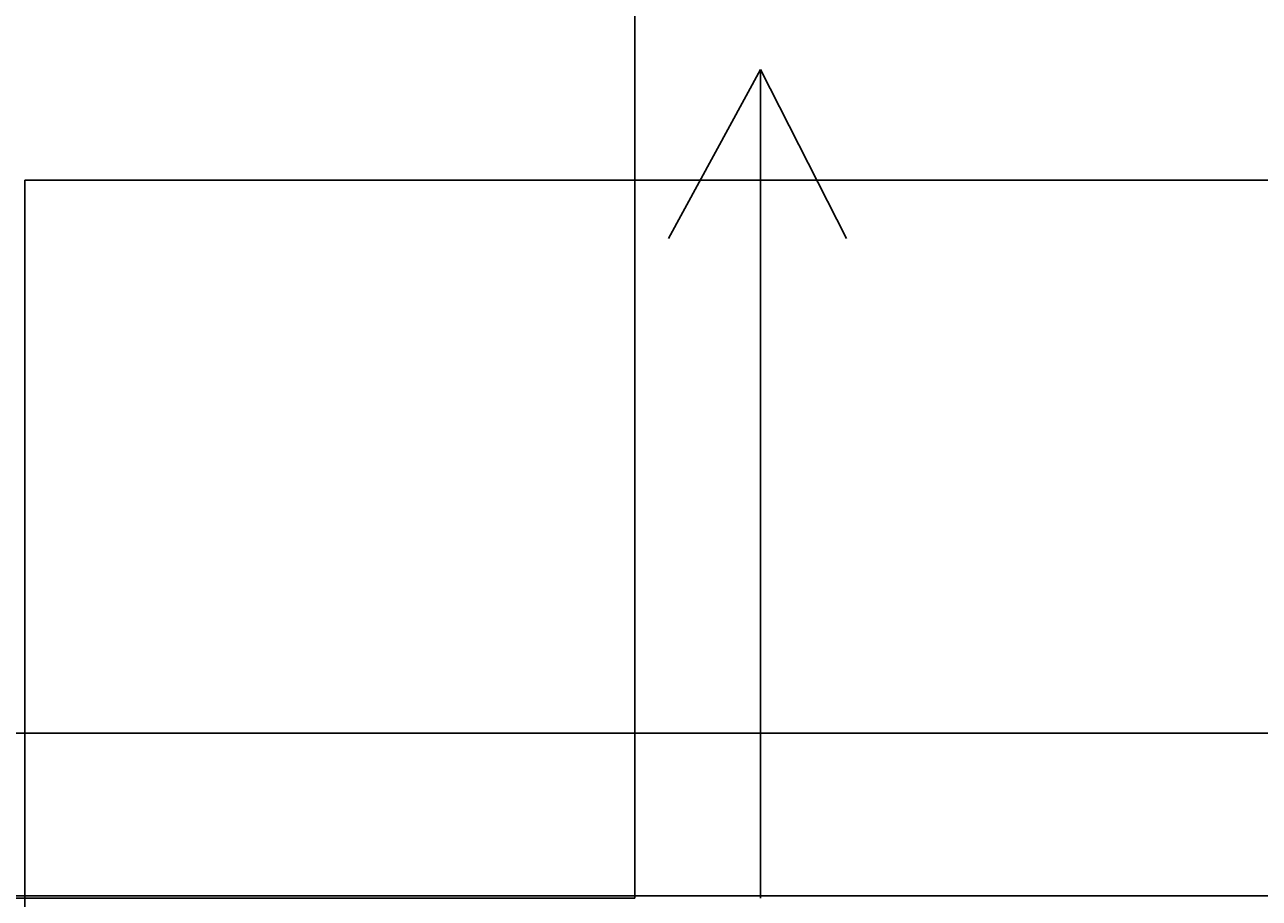
# Model space of a CAD drawing. Units: inches. Extents: x 35362 to 73946, y 43607 to 67532.
# Tile 134 of 134: x 67327 to 69338, y 60122 to 61547. Entities that reach past the tile are written whole.
import ezdxf

# ---------------------------------------------------------------- set-up
doc = ezdxf.new("R2010")
doc.units = ezdxf.units.IN
doc.header["$MEASUREMENT"] = 0
doc.layers.add('A-ANNO-DIMS', color=2, linetype='Continuous', lineweight=18)
doc.layers.add('E-SYMB', color=1, linetype='Continuous', lineweight=25)
doc.styles.get("Standard").update_dxf_attribs({"font": 'arial.ttf'})
doc.dimstyles.get("Standard").update_dxf_attribs({"dimtxt": 0.18, "dimasz": 0.18, "dimexe": 0.18, "dimexo": 0.0625, "dimgap": 0.09, "dimtad": 0, "dimtih": 1, "dimtoh": 1, "dimdec": 4, "dimzin": 0, "dimdsep": 46, "dimtxsty": 'Standard', "dimcen": 0.09, "dimadec": 0, "dimazin": 0, "dimtfac": 1, "dimtdec": 4, "dimtofl": 0, "dimtmove": 0, "dimatfit": 3, "dimfxl": 1, "dimtolj": 1, "dimtzin": 0, "dimarcsym": 0})

# ---------------------------------------------------------------- blocks, each defined once
blk = doc.blocks.new('PWR-5V')
for p, q in [((149.83075954589, 1350.920325582869), (-0.0001436721213395, 1075.898385659784)), ((149.83075954589, 833.0941938853575), (149.83075954589, 1350.920325582869)), ((289.9554714129044, 1075.898385659784), (149.83075954589, 1350.920325582869)), ((149.83075954589, 416.3126341884199), (149.83075954589, 833.0941938853575)), ((149.83075954589, 416.3126341884199), (149.83075954589, 0.0003315384019515))]:
    blk.add_line(p, q)
blk = doc.blocks.new('*D8')
at = {"layer": 'A-ANNO-DIMS', "color": 0, "lineweight": -2, "transparency": 16777216}
for p, q in [((66271.28651900003, 65771.51172800003), (73945.82566600003, 65771.51172800003)), ((73945.64566600005, 65771.33172800003), (73945.64566600005, 59737.03093663782)), ((73945.64566600005, 53702.36633900002), (73945.64566600005, 59736.66713036224)), ((72185.70816600003, 53702.18633900003), (73945.82566600003, 53702.18633900003))]:
    blk.add_line(p, q, dxfattribs=at)
at = {"layer": 'A-ANNO-DIMS', "color": 0, "transparency": 16777216}
for points in [[(73945.61566600006, 65771.33172800003), (73945.67566600005, 65771.33172800003), (73945.64566600005, 65771.51172800003)], [(73945.61566600006, 53702.36633900002), (73945.67566600005, 53702.36633900002), (73945.64566600005, 53702.18633900003)]]:
    blk.add_solid(points, dxfattribs=at)
at = {"layer": 'Defpoints', "color": 0, "transparency": 16777216}
for p in [(66271.22401900003, 65771.51172800003), (73945.64566600005, 65771.51172800003), (72185.64566600003, 53702.18633900003)]:
    blk.add_point(p, dxfattribs=at)
at = {"layer": 'A-ANNO-DIMS', "color": 0, "transparency": 16777216, "insert": (73945.64566600005, 59736.84903349999), "char_height": 0.18, "attachment_point": 5}
blk.add_mtext('\\A1;12069', dxfattribs=at)
blk = doc.blocks.new('*D35')
at = {"layer": 'A-ANNO-DIMS', "color": 0, "lineweight": -2, "transparency": 16777216}
for p, q in [((61240.907336, 59185.206457), (61240.907336, 67531.691728)), ((61241.08733599999, 67531.51172799998), (64780.42646373397, 67531.51172799998)), ((68320.69076200001, 67531.51172799998), (64781.35163426603, 67531.51172799998)), ((68320.870762, 60122.408832), (68320.870762, 67531.691728))]:
    blk.add_line(p, q, dxfattribs=at)
at = {"layer": 'A-ANNO-DIMS', "color": 0, "transparency": 16777216}
for points in [[(61241.08733599999, 67531.541728), (61241.08733599999, 67531.481728), (61240.907336, 67531.51172799998)], [(68320.69076200001, 67531.541728), (68320.69076200001, 67531.481728), (68320.870762, 67531.51172799998)]]:
    blk.add_solid(points, dxfattribs=at)
at = {"layer": 'Defpoints', "color": 0, "transparency": 16777216}
for p in [(68320.870762, 67531.51172799998), (68320.870762, 60122.346332), (61240.907336, 59185.14395699999)]:
    blk.add_point(p, dxfattribs=at)
at = {"layer": 'A-ANNO-DIMS', "color": 0, "transparency": 16777216, "insert": (64780.889049, 67531.51172799998), "char_height": 0.18, "attachment_point": 5}
blk.add_mtext('\\A1;7080.0', dxfattribs=at)
blk = doc.blocks.new('*D36')
at = {"layer": 'A-ANNO-DIMS', "color": 0, "lineweight": -2, "transparency": 16777216}
for p, q in [((68320.80826200004, 60122.34633200002), (35361.76908500003, 60122.34633200002)), ((35361.94908500003, 60122.16633200002), (35361.94908500003, 57247.82893113781)), ((35361.94908500003, 54373.12772400002), (35361.94908500003, 57247.46512486223)), ((68320.80826200004, 54372.94772400003), (35361.76908500003, 54372.94772400002))]:
    blk.add_line(p, q, dxfattribs=at)
at = {"layer": 'A-ANNO-DIMS', "color": 0, "transparency": 16777216}
for points in [[(35361.91908500003, 60122.16633200002), (35361.97908500003, 60122.16633200002), (35361.94908500003, 60122.34633200002)], [(35361.91908500003, 54373.12772400002), (35361.97908500003, 54373.12772400002), (35361.94908500003, 54372.94772400002)]]:
    blk.add_solid(points, dxfattribs=at)
at = {"layer": 'Defpoints', "color": 0, "transparency": 16777216}
for p in [(68320.87076200004, 60122.34633200002), (35361.94908500003, 54372.94772400002), (68320.87076200004, 54372.94772400003)]:
    blk.add_point(p, dxfattribs=at)
at = {"layer": 'A-ANNO-DIMS', "color": 0, "transparency": 16777216, "insert": (35361.94908500004, 57247.64702799999), "char_height": 0.18, "attachment_point": 5}
blk.add_mtext('\\A1;5749.4', dxfattribs=at)
blk = doc.blocks.new('*D65')
at = {"layer": 'A-ANNO-DIMS', "color": 0, "lineweight": -2, "transparency": 16777216}
for p, q in [((65336.01600799999, 61293.223552), (65336.01600799999, 43606.678996)), ((67326.639741, 61293.223552), (67326.639741, 43606.678996)), ((65336.19600799999, 43606.858996), (66330.87277900206, 43606.858996)), ((67326.45974100001, 43606.858996), (66331.78296999796, 43606.858996))]:
    blk.add_line(p, q, dxfattribs=at)
at = {"layer": 'A-ANNO-DIMS', "color": 0, "transparency": 16777216}
for points in [[(65336.19600799999, 43606.888996), (65336.19600799999, 43606.828996), (65336.01600799999, 43606.858996)], [(67326.45974100001, 43606.888996), (67326.45974100001, 43606.828996), (67326.639741, 43606.858996)]]:
    blk.add_solid(points, dxfattribs=at)
at = {"layer": 'Defpoints', "color": 0, "transparency": 16777216}
for p in [(65336.01600799999, 61293.286052), (67326.639741, 61293.286052), (67326.639741, 43606.858996)]:
    blk.add_point(p, dxfattribs=at)
at = {"layer": 'A-ANNO-DIMS', "color": 0, "transparency": 16777216, "insert": (66331.32787450001, 43606.858996), "char_height": 0.18, "attachment_point": 5}
blk.add_mtext('\\A1;1990.6', dxfattribs=at)
blk = doc.blocks.new('*D66')
at = {"layer": 'A-ANNO-DIMS', "color": 0, "lineweight": -2, "transparency": 16777216}
for p, q in [((67326.70224100004, 64127.44160800003), (73945.82566600003, 64127.44160800003)), ((73945.64566600005, 64127.26160800003), (73945.64566600005, 62710.54579452936)), ((73945.64566600005, 61293.46605200003), (73945.64566600005, 62710.1818654707)), ((67326.70224100004, 61293.28605200003), (73945.82566600003, 61293.28605200003))]:
    blk.add_line(p, q, dxfattribs=at)
at = {"layer": 'A-ANNO-DIMS', "color": 0, "transparency": 16777216}
for points in [[(73945.61566600006, 64127.26160800003), (73945.67566600005, 64127.26160800003), (73945.64566600005, 64127.44160800003)], [(73945.61566600006, 61293.46605200003), (73945.67566600005, 61293.46605200003), (73945.64566600005, 61293.28605200003)]]:
    blk.add_solid(points, dxfattribs=at)
at = {"layer": 'Defpoints', "color": 0, "transparency": 16777216}
for p in [(67326.63974100004, 64127.44160800003), (73945.64566600005, 64127.44160800003), (67326.63974100004, 61293.28605200003)]:
    blk.add_point(p, dxfattribs=at)
at = {"layer": 'A-ANNO-DIMS', "color": 0, "transparency": 16777216, "insert": (73945.64566600005, 62710.36383), "char_height": 0.18, "attachment_point": 5}
blk.add_mtext('\\A1;2834.2', dxfattribs=at)
blk = doc.blocks.new('*D69')
at = {"layer": 'A-ANNO-DIMS', "color": 0, "lineweight": -2, "transparency": 16777216}
for p, q in [((68320.870762, 60122.408832), (68320.870762, 67531.691728)), ((68321.050762, 67531.51172799998), (69913.30289879469, 67531.51172799998)), ((71506.482539, 67531.51172799998), (69914.23040220531, 67531.51172799998)), ((71506.662539, 59451.647447), (71506.662539, 67531.691728))]:
    blk.add_line(p, q, dxfattribs=at)
at = {"layer": 'A-ANNO-DIMS', "color": 0, "transparency": 16777216}
for points in [[(68321.050762, 67531.541728), (68321.050762, 67531.481728), (68320.870762, 67531.51172799998)], [(71506.482539, 67531.541728), (71506.482539, 67531.481728), (71506.662539, 67531.51172799998)]]:
    blk.add_solid(points, dxfattribs=at)
at = {"layer": 'Defpoints', "color": 0, "transparency": 16777216}
for p in [(71506.662539, 67531.51172799998), (68320.870762, 60122.346332), (71506.662539, 59451.584947)]:
    blk.add_point(p, dxfattribs=at)
at = {"layer": 'A-ANNO-DIMS', "color": 0, "transparency": 16777216, "insert": (69913.76665050001, 67531.51172799998), "char_height": 0.18, "attachment_point": 5}
blk.add_mtext('\\A1;3185.8', dxfattribs=at)
blk = doc.blocks.new('*D70')
at = {"layer": 'A-ANNO-DIMS', "color": 0, "lineweight": -2, "transparency": 16777216}
for p, q in [((60785.27513900002, 64923.75242000003), (73945.82566600003, 64923.75242000003)), ((73945.64566600005, 64923.57242000003), (73945.64566600005, 62054.63015302935)), ((73945.64566600005, 59185.32395700003), (73945.64566600005, 62054.26622397069)), ((61240.96983600002, 59185.14395700003), (73945.82566600003, 59185.14395700003))]:
    blk.add_line(p, q, dxfattribs=at)
at = {"layer": 'A-ANNO-DIMS', "color": 0, "transparency": 16777216}
for points in [[(73945.61566600006, 64923.57242000003), (73945.67566600005, 64923.57242000003), (73945.64566600005, 64923.75242000003)], [(73945.61566600006, 59185.32395700003), (73945.67566600005, 59185.32395700003), (73945.64566600005, 59185.14395700003)]]:
    blk.add_solid(points, dxfattribs=at)
at = {"layer": 'Defpoints', "color": 0, "transparency": 16777216}
for p in [(60785.21263900002, 64923.75242000003), (73945.64566600005, 64923.75242000003), (61240.90733600002, 59185.14395700003)]:
    blk.add_point(p, dxfattribs=at)
at = {"layer": 'A-ANNO-DIMS', "color": 0, "transparency": 16777216, "insert": (73945.64566600005, 62054.44818849999), "char_height": 0.18, "attachment_point": 5}
blk.add_mtext('\\A1;5738.6', dxfattribs=at)
blk = doc.blocks.new('*D71')
at = {"layer": 'A-ANNO-DIMS', "color": 0, "lineweight": -2, "transparency": 16777216}
for p, q in [((63159.24181700003, 64828.55626700002), (73945.82566600003, 64828.55626700002)), ((73945.64566600005, 64828.37626700002), (73945.64566600005, 62007.03207652936)), ((73945.64566600005, 59185.32395700003), (73945.64566600005, 62006.6681474707)), ((61240.96983600002, 59185.14395700003), (73945.82566600003, 59185.14395700003))]:
    blk.add_line(p, q, dxfattribs=at)
at = {"layer": 'A-ANNO-DIMS', "color": 0, "transparency": 16777216}
for points in [[(73945.61566600006, 64828.37626700002), (73945.67566600005, 64828.37626700002), (73945.64566600005, 64828.55626700002)], [(73945.61566600006, 59185.32395700003), (73945.67566600005, 59185.32395700003), (73945.64566600005, 59185.14395700003)]]:
    blk.add_solid(points, dxfattribs=at)
at = {"layer": 'Defpoints', "color": 0, "transparency": 16777216}
for p in [(63159.17931700003, 64828.55626700002), (73945.64566600005, 64828.55626700002), (61240.90733600002, 59185.14395700003)]:
    blk.add_point(p, dxfattribs=at)
at = {"layer": 'A-ANNO-DIMS', "color": 0, "transparency": 16777216, "insert": (73945.64566600005, 62006.85011199999), "char_height": 0.18, "attachment_point": 5}
blk.add_mtext('\\A1;5643.4', dxfattribs=at)
blk = doc.blocks.new('*D113')
at = {"layer": 'A-ANNO-DIMS', "color": 0, "lineweight": -2, "transparency": 16777216}
for p, q in [((53526.13474100003, 60391.71935800003), (73945.82566600003, 60391.71935800003)), ((73945.64566600005, 60391.53935800003), (73945.64566600005, 60259.19182863781)), ((73945.64566600005, 60126.48049300003), (73945.64566600005, 60258.82802236224)), ((53705.42262200003, 60126.30049300003), (73945.82566600003, 60126.30049300003))]:
    blk.add_line(p, q, dxfattribs=at)
at = {"layer": 'A-ANNO-DIMS', "color": 0, "transparency": 16777216}
for points in [[(73945.61566600006, 60391.53935800003), (73945.67566600005, 60391.53935800003), (73945.64566600005, 60391.71935800003)], [(73945.61566600006, 60126.48049300003), (73945.67566600005, 60126.48049300003), (73945.64566600005, 60126.30049300003)]]:
    blk.add_solid(points, dxfattribs=at)
at = {"layer": 'Defpoints', "color": 0, "transparency": 16777216}
for p in [(53526.07224100003, 60391.71935800003), (73945.64566600005, 60391.71935800003), (53705.36012200003, 60126.30049300003)]:
    blk.add_point(p, dxfattribs=at)
at = {"layer": 'A-ANNO-DIMS', "color": 0, "transparency": 16777216, "insert": (73945.64566600005, 60259.00992549999), "char_height": 0.18, "attachment_point": 5}
blk.add_mtext('\\A1;265.4', dxfattribs=at)

msp = doc.modelspace()

# ---------------------------------------------------------------- block references
at = {"layer": 'E-SYMB'}
msp.add_blockref('PWR-5V', (68375.605, 60122.346), dxfattribs=at)

# ---------------------------------------------------------------- dimensions: what is measured, and where the dimension line sits
at = {"layer": 'A-ANNO-DIMS'}
for base, p1, p2, picture, middle in [((68320.870762, 67531.51172799998), (61240.907336, 59185.14395699999), (68320.870762, 60122.346332), '*D35', (64780.889049, 67531.51172799998)), ((71506.662539, 67531.51172799998), (68320.870762, 60122.346332), (71506.662539, 59451.584947), '*D69', (69913.76665050001, 67531.51172799998)), ((67326.639741, 43606.858996), (65336.01600799999, 61293.286052), (67326.639741, 61293.286052), '*D65', (66331.32787450001, 43606.858996))]:
    dim = msp.add_linear_dim(base=base, p1=p1, p2=p2, dimstyle='Standard', override={"dimdec": 1, "dimlfac": 1, "dimrnd": 0, "dimzin": 0, "dimdsep": 46, "dimlunit": 2}, dxfattribs=at)
    dim.commit()
    dim.dimension.update_dxf_attribs({"geometry": picture, "text_midpoint": middle})
for base, p1, p2, override, picture, middle in [((73945.64566600005, 65771.51172800003), (72185.645666, 53702.186339), (66271.224019, 65771.51172799998), {"dimdec": 0, "dimlfac": 1, "dimrnd": 0, "dimzin": 0, "dimdsep": 46, "dimlunit": 2}, '*D8', (73945.64566600005, 59736.84903349999)), ((73945.64566600005, 64923.75242000003), (61240.907336, 59185.14395699999), (60785.21263899999, 64923.75241999999), {"dimdec": 1, "dimlfac": 1, "dimrnd": 0, "dimzin": 0, "dimdsep": 46, "dimlunit": 2}, '*D70', (73945.64566600005, 62054.44818849999)), ((73945.64566600005, 64828.55626700002), (61240.907336, 59185.14395699999), (63159.179317, 64828.556267), {"dimdec": 1, "dimlfac": 1, "dimrnd": 0, "dimzin": 0, "dimdsep": 46, "dimlunit": 2}, '*D71', (73945.64566600005, 62006.85011199999)), ((73945.64566600005, 64127.44160800003), (67326.639741, 61293.286052), (67326.639741, 64127.44160799999), {"dimdec": 1, "dimlfac": 1, "dimrnd": 0, "dimzin": 0, "dimdsep": 46, "dimlunit": 2}, '*D66', (73945.64566600005, 62710.36383)), ((73945.64566600005, 60391.71935800003), (53705.36012199999, 60126.300493), (53526.072241, 60391.719358), {"dimdec": 1, "dimlfac": 1, "dimrnd": 0, "dimzin": 0, "dimdsep": 46, "dimlunit": 2}, '*D113', (73945.64566600005, 60259.00992549999)), ((35361.94908500003, 54372.94772400002), (68320.870762, 60122.346332), (68320.870762, 54372.947724), {"dimdec": 1, "dimlfac": 1, "dimrnd": 0, "dimzin": 0, "dimdsep": 46, "dimlunit": 2}, '*D36', (35361.94908500004, 57247.64702799999))]:
    dim = msp.add_linear_dim(base=base, p1=p1, p2=p2, angle=90, dimstyle='Standard', override=override, dxfattribs=at)
    dim.commit()
    dim.dimension.update_dxf_attribs({"geometry": picture, "text_midpoint": middle})

doc.saveas('drawing.dxf')
